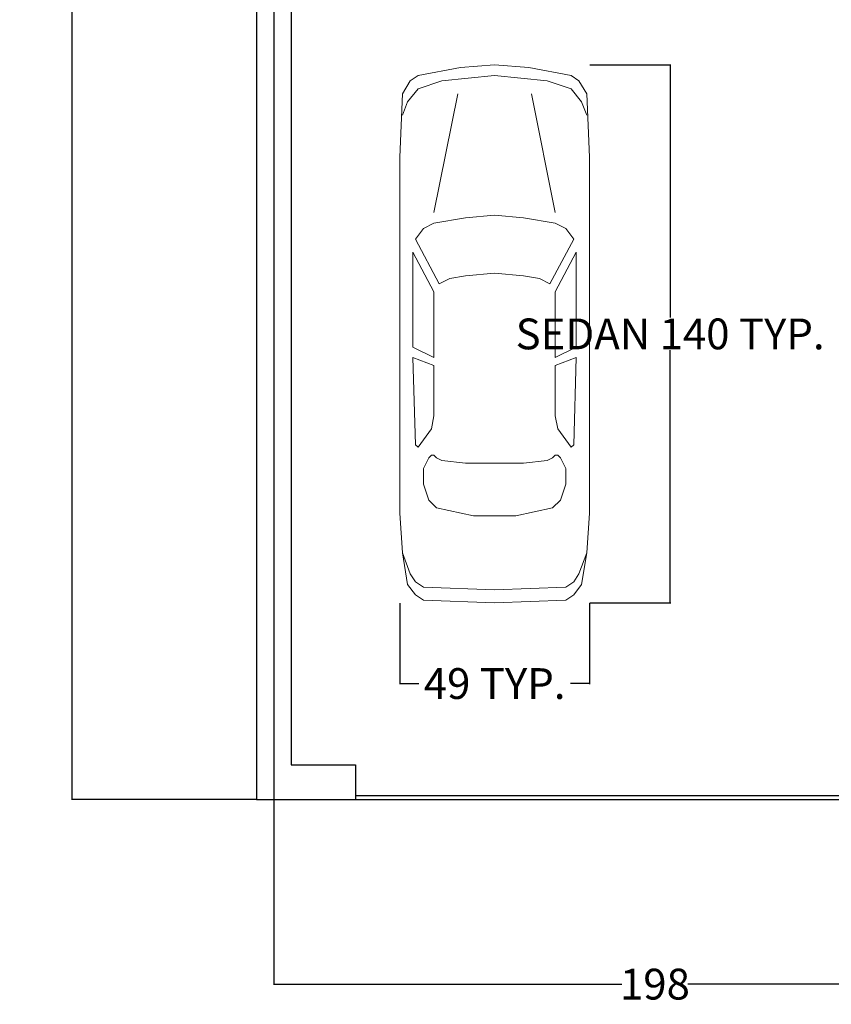
# Model space of a CAD drawing. Units: inches. Extents: x -48 to 50072, y 0 to 21068.
# Tile 2 of 75: x -48 to 163, y 161 to 417. Entities that reach past the tile are written whole.
import ezdxf

# ---------------------------------------------------------------- set-up
doc = ezdxf.new("R2010")
doc.units = ezdxf.units.IN
doc.header["$MEASUREMENT"] = 0
doc.linetypes.add('ACAD_ISO02W100', pattern=[15, 12, -3])
for name, color, linetype, lineweight in [('A-ANNO-DIMS', 2, 'Continuous', 18), ('C-PROP', 7, 'Continuous', 25), ('C-PROP-REF', 32, 'ACAD_ISO02W100', 13), ('C-SITE-VEHC', 8, 'Continuous', 13)]:
    doc.layers.add(name, color=color, linetype=linetype, lineweight=lineweight)
doc.styles.get("Standard").update_dxf_attribs({"font": 'arial.ttf'})
doc.dimstyles.get("Standard").update_dxf_attribs({"dimtxt": 8, "dimasz": 0.18, "dimexe": 0.18, "dimexo": 0.0625, "dimgap": 0.09, "dimtad": 0, "dimtih": 1, "dimtoh": 1, "dimdec": 1, "dimzin": 0, "dimdsep": 46, "dimlunit": 4, "dimtxsty": 'Standard', "dimblk": 'ARCHTICK', "dimcen": 0.09, "dimadec": 0, "dimazin": 0, "dimtfac": 1, "dimtdec": 1, "dimtofl": 0, "dimtmove": 0, "dimatfit": 3, "dimldrblk": 'ARCHTICK', "dimfxl": 1, "dimtolj": 1, "dimtzin": 0, "dimarcsym": 0})

# ---------------------------------------------------------------- blocks, each defined once
blk = doc.blocks.new('CAR-PLAN-SEDAN')
for p, q in [((15.75, 139.03), (4.79, 136.97)), ((24.65, 139.71), (15.75, 139.03)), ((24.65, 139.71), (33.56, 139.03)), ((33.56, 139.03), (44.52, 136.97)), ((2.74, 135.6), (0.68, 132.18)), ((4.79, 136.97), (2.74, 135.6)), ((10.96, 135.6), (4.79, 133.55)), ((24.65, 136.97), (10.96, 135.6)), ((24.65, 136.97), (38.35, 135.6)), ((38.35, 135.6), (44.52, 133.55)), ((44.52, 136.97), (46.57, 135.6)), ((46.57, 135.6), (48.62, 132.18)), ((4.79, 133.55), (2.05, 130.12)), ((44.52, 133.55), (47.25, 130.12)), ((0.68, 132.18), (0, 115.74)), ((15.07, 132.18), (8.9, 101.36)), ((34.24, 132.18), (40.41, 101.36)), ((48.62, 132.18), (49.31, 115.74)), ((2.05, 130.12), (0.68, 126.7)), ((47.25, 130.12), (48.62, 126.7)), ((0, 115.74), (0, 23.29)), ((49.31, 115.74), (49.31, 23.29)), ((17.12, 99.99), (8.9, 98.62)), ((24.65, 100.67), (17.12, 99.99)), ((24.65, 100.67), (32.19, 99.99)), ((32.19, 99.99), (40.41, 98.62)), ((6.16, 97.25), (4.11, 94.51)), ((8.9, 98.62), (6.16, 97.25)), ((40.41, 98.62), (43.15, 97.25)), ((43.15, 97.25), (45.2, 94.51)), ((4.11, 94.51), (10.27, 82.87)), ((45.2, 94.51), (39.04, 82.87)), ((3.42, 91.09), (8.9, 80.81)), ((3.42, 66.43), (3.42, 91.09)), ((45.88, 91.09), (40.41, 80.81)), ((45.88, 66.43), (45.88, 91.09)), ((13.01, 84.24), (17.12, 84.92)), ((17.12, 84.92), (24.65, 85.61)), ((32.19, 84.92), (24.65, 85.61)), ((36.3, 84.24), (32.19, 84.92)), ((10.27, 82.87), (13.01, 84.24)), ((39.04, 82.87), (36.3, 84.24)), ((8.9, 80.81), (8.9, 63.69)), ((40.41, 80.81), (40.41, 63.69)), ((8.9, 63.69), (3.42, 66.43)), ((40.41, 63.69), (45.88, 66.43)), ((4.11, 41.09), (3.42, 63.69)), ((3.42, 63.69), (8.9, 61.64)), ((8.9, 61.64), (8.9, 48.62)), ((45.88, 63.69), (40.41, 61.64)), ((40.41, 61.64), (40.41, 48.62)), ((45.2, 41.09), (45.88, 63.69)), ((8.9, 48.62), (8.22, 45.2)), ((40.41, 48.62), (41.09, 45.2)), ((8.22, 45.2), (4.79, 40.41)), ((41.09, 45.2), (44.52, 40.41)), ((4.79, 40.41), (4.11, 41.09)), ((44.52, 40.41), (45.2, 41.09)), ((7.53, 37.67), (6.16, 34.93)), ((8.22, 38.35), (7.53, 37.67)), ((8.9, 38.35), (8.22, 38.35)), ((9.59, 37.67), (8.9, 38.35)), ((10.96, 36.98), (9.59, 37.67)), ((17.12, 36.3), (10.96, 36.98)), ((24.65, 36.3), (17.12, 36.3)), ((24.65, 36.3), (32.19, 36.3)), ((32.19, 36.3), (38.35, 36.98)), ((38.35, 36.98), (39.72, 37.67)), ((39.72, 37.67), (40.41, 38.35)), ((40.41, 38.35), (41.09, 38.35)), ((41.09, 38.35), (41.78, 37.67)), ((41.78, 37.67), (43.15, 34.93)), ((6.16, 34.93), (6.16, 30.82)), ((43.15, 34.93), (43.15, 30.82)), ((6.16, 30.82), (7.53, 26.71)), ((43.15, 30.82), (41.78, 26.71)), ((7.53, 26.71), (9.59, 24.65)), ((41.78, 26.71), (39.72, 24.65)), ((0, 23.29), (0.68, 13.01)), ((9.59, 24.65), (19.18, 22.6)), ((39.72, 24.65), (30.13, 22.6)), ((49.31, 23.29), (48.62, 13.01)), ((19.18, 22.6), (24.65, 22.6)), ((30.13, 22.6), (24.65, 22.6)), ((0.68, 13.01), (2.74, 7.53)), ((0.68, 13.01), (2.05, 4.79)), ((48.62, 13.01), (46.57, 7.53)), ((48.62, 13.01), (47.25, 4.79)), ((2.74, 7.53), (4.11, 5.48)), ((4.11, 5.48), (6.16, 4.11)), ((45.2, 5.48), (43.15, 4.11)), ((46.57, 7.53), (45.2, 5.48)), ((2.05, 4.79), (4.11, 2.05)), ((6.16, 4.11), (24.65, 3.42)), ((43.15, 4.11), (24.65, 3.42)), ((47.25, 4.79), (45.2, 2.05)), ((4.11, 2.05), (6.16, 0.69)), ((6.16, 0.69), (24.65, 0)), ((43.15, 0.69), (24.65, 0)), ((45.2, 2.05), (43.15, 0.69))]:
    blk.add_line(p, q)
blk = doc.blocks.new('_ArchTick')
at = {"color": 0, "linetype": 'ByBlock', "const_width": 0.15}
blk.add_lwpolyline([(-0.5, -0.5), (0.5, 0.5)], dxfattribs=at)
blk = doc.blocks.new('*D96')
at = {"layer": 'A-ANNO-DIMS', "color": 0, "lineweight": -2, "transparency": 16777216}
for p, q in [((100.08, 404.86), (121.15, 404.86)), ((120.97, 404.86), (120.97, 339.23)), ((120.97, 265.15), (120.97, 330.78)), ((100.08, 265.15), (121.15, 265.15))]:
    blk.add_line(p, q, dxfattribs=at)
at = {"layer": 'Defpoints', "color": 0, "transparency": 16777216}
for p in [(100.01, 404.86), (120.97, 404.86), (100.01, 265.15)]:
    blk.add_point(p, dxfattribs=at)
at = {"layer": 'A-ANNO-DIMS', "color": 0, "lineweight": -2, "transparency": 16777216, "xscale": 0.18, "yscale": 0.18, "zscale": 0.18}
for p, rotation in [((120.97, 404.86), 90), ((120.97, 265.15), 270)]:
    blk.add_blockref('_ArchTick', p, dxfattribs=dict(at, rotation=rotation))
at = {"layer": 'A-ANNO-DIMS', "color": 0, "transparency": 16777216, "insert": (120.97, 335.01), "char_height": 8, "attachment_point": 5}
blk.add_mtext('\\A1;SEDAN 140 TYP.', dxfattribs=at)
blk = doc.blocks.new('*D97')
at = {"layer": 'A-ANNO-DIMS', "color": 0, "lineweight": -2, "transparency": 16777216}
for p, q in [((50.7, 265.09), (50.7, 244.01)), ((100.01, 265.09), (100.01, 244.01)), ((50.7, 244.19), (55.64, 244.19)), ((100.01, 244.19), (95.08, 244.19))]:
    blk.add_line(p, q, dxfattribs=at)
at = {"layer": 'Defpoints', "color": 0, "transparency": 16777216}
for p in [(50.7, 265.15), (100.01, 265.15), (100.01, 244.19)]:
    blk.add_point(p, dxfattribs=at)
at = {"layer": 'A-ANNO-DIMS', "color": 0, "lineweight": -2, "transparency": 16777216, "xscale": 0.18, "yscale": 0.18, "zscale": 0.18, "rotation": 180}
blk.add_blockref('_ArchTick', (50.7, 244.19), dxfattribs=at)
at = {"layer": 'A-ANNO-DIMS', "color": 0, "lineweight": -2, "transparency": 16777216, "xscale": 0.18, "yscale": 0.18, "zscale": 0.18}
blk.add_blockref('_ArchTick', (100.01, 244.19), dxfattribs=at)
at = {"layer": 'A-ANNO-DIMS', "color": 0, "transparency": 16777216, "insert": (75.36, 244.19), "char_height": 8, "attachment_point": 5}
blk.add_mtext('\\A1;49 TYP.', dxfattribs=at)
blk = doc.blocks.new('*D113')
at = {"layer": 'A-ANNO-DIMS', "color": 0, "lineweight": -2, "transparency": 16777216}
for p, q in [((13.45, 1170.77), (-34.61, 1170.77)), ((-34.43, 1170.77), (-34.43, 696.6)), ((-34.43, 214.07), (-34.43, 688.25)), ((13.45, 214.07), (-34.61, 214.07))]:
    blk.add_line(p, q, dxfattribs=at)
at = {"layer": 'Defpoints', "color": 0, "transparency": 16777216}
for p in [(-34.43, 1170.77), (13.52, 1170.77), (13.52, 214.07)]:
    blk.add_point(p, dxfattribs=at)
at = {"layer": 'A-ANNO-DIMS', "color": 0, "lineweight": -2, "transparency": 16777216, "xscale": 0.18, "yscale": 0.18, "zscale": 0.18}
for p, rotation in [((-34.43, 1170.77), 90), ((-34.43, 214.07), 270)]:
    blk.add_blockref('_ArchTick', p, dxfattribs=dict(at, rotation=rotation))
at = {"layer": 'A-ANNO-DIMS', "color": 0, "transparency": 16777216, "insert": (-34.43, 692.42), "char_height": 8, "attachment_point": 5}
blk.add_mtext('\\A1;956.7', dxfattribs=at)
blk = doc.blocks.new('*D116')
at = {"layer": 'A-ANNO-DIMS', "color": 0, "lineweight": -2, "transparency": 16777216}
for p, q in [((18.02, 677.71), (18.02, 165.94)), ((216.02, 677.71), (216.02, 165.94)), ((18.02, 166.12), (108.46, 166.12)), ((216.02, 166.12), (125.58, 166.12))]:
    blk.add_line(p, q, dxfattribs=at)
at = {"layer": 'Defpoints', "color": 0, "transparency": 16777216}
for p in [(18.02, 677.77), (216.02, 677.77), (216.02, 166.12)]:
    blk.add_point(p, dxfattribs=at)
at = {"layer": 'A-ANNO-DIMS', "color": 0, "lineweight": -2, "transparency": 16777216, "xscale": 0.18, "yscale": 0.18, "zscale": 0.18, "rotation": 180}
blk.add_blockref('_ArchTick', (18.02, 166.12), dxfattribs=at)
at = {"layer": 'A-ANNO-DIMS', "color": 0, "lineweight": -2, "transparency": 16777216, "xscale": 0.18, "yscale": 0.18, "zscale": 0.18}
blk.add_blockref('_ArchTick', (216.02, 166.12), dxfattribs=at)
at = {"layer": 'A-ANNO-DIMS', "color": 0, "transparency": 16777216, "insert": (117.02, 166.12), "char_height": 8, "attachment_point": 5}
blk.add_mtext('\\A1;198', dxfattribs=at)

msp = doc.modelspace()

# ---------------------------------------------------------------- linework, layer by layer
at = {"layer": 'C-PROP'}
for p, q in [((13.517, 1170.775), (13.517, 214.075)), ((22.517, 860.775), (22.517, 223.075)), ((22.517, 223.075), (39.243, 223.075)), ((39.243, 223.075), (39.243, 214.075)), ((39.243, 215.075), (165.389, 215.075)), ((13.517, 214.075), (39.243, 214.075)), ((39.243, 214.075), (165.389, 214.075))]:
    msp.add_line(p, q, dxfattribs=at)
at = {"layer": 'C-PROP-REF'}
msp.add_line((18.017, 1166.275), (18.017, 214.075), dxfattribs=at)

# ---------------------------------------------------------------- block references
at = {"layer": 'C-SITE-VEHC'}
msp.add_blockref('CAR-PLAN-SEDAN', (50.705, 265.15), dxfattribs=at)

# ---------------------------------------------------------------- dimensions: what is measured, and where the dimension line sits
at = {"layer": 'A-ANNO-DIMS'}
dim = msp.add_linear_dim(base=(-34.433, 1170.775), p1=(13.517, 214.075), p2=(13.517, 1170.775), angle=90, dimstyle='Standard', override={"dimdec": 1, "dimlfac": 1, "dimrnd": 0, "dimzin": 0, "dimdsep": 46, "dimlunit": 2}, dxfattribs=at)
dim.commit()
dim.dimension.update_dxf_attribs({"geometry": '*D113', "text_midpoint": (-34.433, 692.425)})
dim = msp.add_linear_dim(base=(216.017, 166.125), p1=(18.017, 677.775), p2=(216.017, 677.775), dimstyle='Standard', override={"dimdec": 0, "dimlfac": 1, "dimrnd": 0, "dimzin": 0, "dimdsep": 46, "dimlunit": 2}, dxfattribs=at)
dim.commit()
dim.dimension.update_dxf_attribs({"geometry": '*D116', "text_midpoint": (117.017, 166.125)})
dim = msp.add_linear_dim(base=(120.971, 404.86), p1=(100.014, 265.15), p2=(100.014, 404.86), angle=90, text='SEDAN <> TYP.', dimstyle='Standard', override={"dimdec": 0, "dimlfac": 1, "dimrnd": 0, "dimzin": 0, "dimdsep": 46, "dimlunit": 2}, dxfattribs=at)
dim.commit()
dim.dimension.update_dxf_attribs({"geometry": '*D96', "text_midpoint": (120.971, 335.005)})
dim = msp.add_linear_dim(base=(100.014, 244.194), p1=(50.705, 265.15), p2=(100.014, 265.15), text='<> TYP.', dimstyle='Standard', override={"dimdec": 0, "dimlfac": 1, "dimrnd": 0, "dimzin": 0, "dimdsep": 46, "dimlunit": 2}, dxfattribs=at)
dim.commit()
dim.dimension.update_dxf_attribs({"geometry": '*D97', "text_midpoint": (75.36, 244.194)})

doc.saveas('drawing.dxf')
